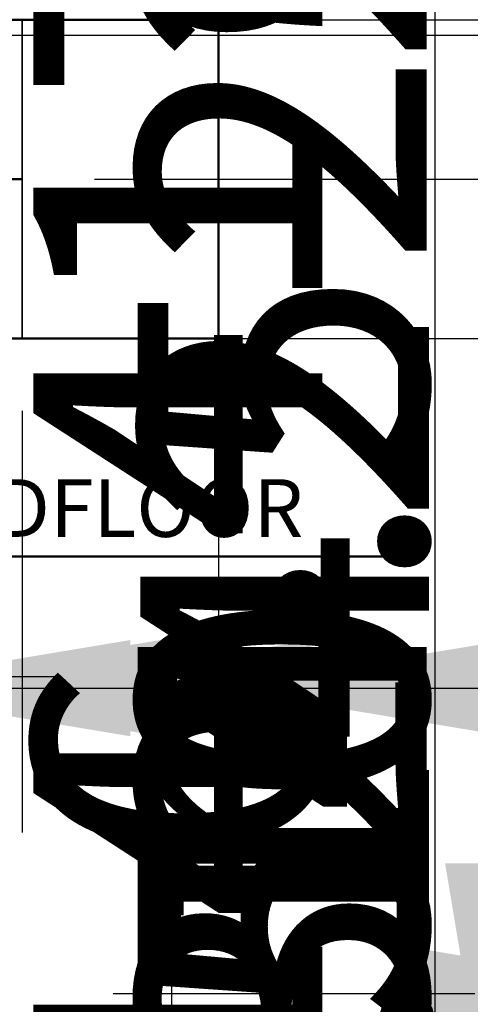
# Model space of a CAD drawing. Units: metres. Extents: x 782 to 1487, y 1262 to 7446.
# Tile 10 of 25: x 830.694 to 834.592, y 1284.539 to 1293.067. Entities that reach past the tile are written whole.
import ezdxf

# ---------------------------------------------------------------- set-up
doc = ezdxf.new("R2010")
doc.units = ezdxf.units.M
for name, color, linetype, lineweight in [('A-ANNO-DIMS', 2, 'Continuous', 18), ('A-ANNO-TEXT', 3, 'Continuous', 18), ('A-FLOR-STRS', 3, 'Continuous', 25), ('A-WALL', 7, 'Continuous', 50)]:
    doc.layers.add(name, color=color, linetype=linetype, lineweight=lineweight)
doc.styles.get("Standard").update_dxf_attribs({"font": 'arial.ttf'})
doc.dimstyles.new('ISO-25', dxfattribs={"dimtxt": 2.5, "dimasz": 2.5, "dimexe": 1.25, "dimexo": 0.625, "dimtad": 1, "dimtxsty": 'Standard', "dimcen": 2.5, "dimadec": 0, "dimazin": 0, "dimtfac": 1, "dimtmove": 0, "dimatfit": 3, "dimfxl": 1, "dimarcsym": 0})

# ---------------------------------------------------------------- blocks, each defined once
blk = doc.blocks.new('*D6')
at = {"layer": 'A-ANNO-DIMS', "color": 0, "lineweight": -2, "transparency": 16777216}
for p, q in [((833.0375, 1307.3274), (836.7683, 1307.3274)), ((835.5183, 1304.8274), (835.5183, 1295.5674)), ((833.0375, 1293.0674), (836.7683, 1293.0674))]:
    blk.add_line(p, q, dxfattribs=at)
at = {"layer": 'A-ANNO-DIMS', "color": 0, "transparency": 16777216}
for points in [[(835.1017, 1304.8274), (835.935, 1304.8274), (835.5183, 1307.3274)], [(835.1017, 1295.5674), (835.935, 1295.5674), (835.5183, 1293.0674)]]:
    blk.add_solid(points, dxfattribs=at)
at = {"layer": 'Defpoints', "color": 0, "transparency": 16777216}
for p in [(832.4125, 1307.3274), (832.4125, 1293.0674), (835.5183, 1293.0674)]:
    blk.add_point(p, dxfattribs=at)
at = {"layer": 'A-ANNO-DIMS', "color": 0, "transparency": 16777216, "insert": (833.3909, 1300.1974), "char_height": 2.5, "attachment_point": 5, "rotation": 90}
blk.add_mtext('14,26', dxfattribs=at)
blk = doc.blocks.new('*D22')
at = {"layer": 'A-ANNO-DIMS', "color": 0, "lineweight": -2, "transparency": 16777216}
for p, q in [((812.7897, 1292.934), (810.2897, 1292.934)), ((815.2897, 1292.934), (816.1792, 1292.934)), ((818.6792, 1292.934), (848.8344, 1292.934)), ((815.2897, 1292.4424), (815.2897, 1291.684)), ((816.1792, 1292.4424), (816.1792, 1291.684))]:
    blk.add_line(p, q, dxfattribs=at)
at = {"layer": 'A-ANNO-DIMS', "color": 0, "transparency": 16777216}
for points in [[(812.7897, 1293.3507), (812.7897, 1292.5173), (815.2897, 1292.934)], [(818.6792, 1293.3507), (818.6792, 1292.5173), (816.1792, 1292.934)]]:
    blk.add_solid(points, dxfattribs=at)
at = {"layer": 'Defpoints', "color": 0, "transparency": 16777216}
for p in [(815.2897, 1293.0674), (816.1792, 1293.0674), (816.1792, 1292.934)]:
    blk.add_point(p, dxfattribs=at)
at = {"layer": 'A-ANNO-DIMS', "color": 0, "transparency": 16777216, "insert": (835.0068, 1294.8525), "char_height": 2.5, "attachment_point": 5}
blk.add_mtext('DOOR 0.89 TYP.', dxfattribs=at)
blk = doc.blocks.new('*D24')
at = {"layer": 'A-ANNO-DIMS', "color": 0, "lineweight": -2, "transparency": 16777216}
for p, q in [((811.2086, 1294.4231), (808.7086, 1294.4231)), ((813.7086, 1294.4231), (814.5592, 1294.4231)), ((817.0592, 1294.4231), (852.6493, 1294.4231)), ((813.7086, 1293.9257), (813.7086, 1293.1731)), ((814.5592, 1293.9257), (814.5592, 1293.1731))]:
    blk.add_line(p, q, dxfattribs=at)
at = {"layer": 'A-ANNO-DIMS', "color": 0, "transparency": 16777216}
for points in [[(811.2086, 1294.8398), (811.2086, 1294.0065), (813.7086, 1294.4231)], [(817.0592, 1294.8398), (817.0592, 1294.0065), (814.5592, 1294.4231)]]:
    blk.add_solid(points, dxfattribs=at)
at = {"layer": 'Defpoints', "color": 0, "transparency": 16777216}
for p in [(813.7086, 1294.5507), (814.5592, 1294.5507), (814.5592, 1294.4231)]:
    blk.add_point(p, dxfattribs=at)
at = {"layer": 'A-ANNO-DIMS', "color": 0, "transparency": 16777216, "insert": (836.1042, 1296.3416), "char_height": 2.5, "attachment_point": 5}
blk.add_mtext('DOOR D2 0.85 TYP.', dxfattribs=at)
blk = doc.blocks.new('*D76')
at = {"layer": 'A-ANNO-DIMS', "color": 0, "lineweight": -2, "transparency": 16777216}
for p, q in [((814.8832, 1289.6803), (814.8832, 1286.127)), ((816.58, 1289.6803), (816.58, 1286.127)), ((812.3832, 1287.377), (809.8832, 1287.377)), ((814.8832, 1287.377), (816.58, 1287.377)), ((819.08, 1287.377), (831.0309, 1287.377))]:
    blk.add_line(p, q, dxfattribs=at)
at = {"layer": 'A-ANNO-DIMS', "color": 0, "transparency": 16777216}
for points in [[(812.3832, 1287.7936), (812.3832, 1286.9603), (814.8832, 1287.377)], [(819.08, 1287.7936), (819.08, 1286.9603), (816.58, 1287.377)]]:
    blk.add_solid(points, dxfattribs=at)
at = {"layer": 'Defpoints', "color": 0, "transparency": 16777216}
for p in [(814.8832, 1290.3053), (816.58, 1290.3053), (816.58, 1287.377)]:
    blk.add_point(p, dxfattribs=at)
at = {"layer": 'A-ANNO-DIMS', "color": 0, "transparency": 16777216, "insert": (826.3055, 1289.2784), "char_height": 2.5, "attachment_point": 5}
blk.add_mtext('1.697', dxfattribs=at)
blk = doc.blocks.new('*D87')
at = {"layer": 'A-ANNO-DIMS', "color": 0, "lineweight": -2, "transparency": 16777216}
for p, q in [((835.1905, 1309.8274), (835.1905, 1312.3274)), ((833.0375, 1307.3274), (836.4405, 1307.3274)), ((835.1905, 1307.3274), (835.1905, 1304.8669)), ((833.0382, 1304.8669), (836.4405, 1304.8669)), ((835.1905, 1302.3669), (835.1905, 1292.0821))]:
    blk.add_line(p, q, dxfattribs=at)
at = {"layer": 'A-ANNO-DIMS', "color": 0, "transparency": 16777216}
for points in [[(834.7738, 1309.8274), (835.6071, 1309.8274), (835.1905, 1307.3274)], [(834.7738, 1302.3669), (835.6071, 1302.3669), (835.1905, 1304.8669)]]:
    blk.add_solid(points, dxfattribs=at)
at = {"layer": 'Defpoints', "color": 0, "transparency": 16777216}
for p in [(832.4125, 1307.3274), (832.4132, 1304.8669), (835.1905, 1304.8669)]:
    blk.add_point(p, dxfattribs=at)
at = {"layer": 'A-ANNO-DIMS', "color": 0, "transparency": 16777216, "insert": (833.289, 1295.9745), "char_height": 2.5, "attachment_point": 5, "rotation": 90}
blk.add_mtext('2.46', dxfattribs=at)
blk = doc.blocks.new('*D88')
at = {"layer": 'A-ANNO-DIMS', "color": 0, "lineweight": -2, "transparency": 16777216}
for p, q in [((835.1905, 1307.3669), (835.1905, 1309.8669)), ((833.0382, 1304.8669), (836.4405, 1304.8669)), ((835.1905, 1304.8669), (835.1905, 1300.3378)), ((833.0381, 1300.3378), (836.4405, 1300.3378)), ((835.1905, 1297.8378), (835.1905, 1285.5459))]:
    blk.add_line(p, q, dxfattribs=at)
at = {"layer": 'A-ANNO-DIMS', "color": 0, "transparency": 16777216}
for points in [[(834.7738, 1307.3669), (835.6071, 1307.3669), (835.1905, 1304.8669)], [(834.7738, 1297.8378), (835.6071, 1297.8378), (835.1905, 1300.3378)]]:
    blk.add_solid(points, dxfattribs=at)
at = {"layer": 'Defpoints', "color": 0, "transparency": 16777216}
for p in [(832.4132, 1304.8669), (832.4131, 1300.3378), (835.1905, 1300.3378)]:
    blk.add_point(p, dxfattribs=at)
at = {"layer": 'A-ANNO-DIMS', "color": 0, "transparency": 16777216, "insert": (833.289, 1290.4419), "char_height": 2.5, "attachment_point": 5, "rotation": 90}
blk.add_mtext('4.529', dxfattribs=at)
blk = doc.blocks.new('*D89')
at = {"layer": 'A-ANNO-DIMS', "color": 0, "lineweight": -2, "transparency": 16777216}
for p, q in [((835.1905, 1302.8378), (835.1905, 1305.3378)), ((833.0381, 1300.3378), (836.4405, 1300.3378)), ((835.1905, 1300.3378), (835.1905, 1296.196)), ((833.0375, 1296.196), (836.4405, 1296.196)), ((835.1905, 1293.696), (835.1905, 1281.4347))]:
    blk.add_line(p, q, dxfattribs=at)
at = {"layer": 'A-ANNO-DIMS', "color": 0, "transparency": 16777216}
for points in [[(834.7738, 1302.8378), (835.6071, 1302.8378), (835.1905, 1300.3378)], [(834.7738, 1293.696), (835.6071, 1293.696), (835.1905, 1296.196)]]:
    blk.add_solid(points, dxfattribs=at)
at = {"layer": 'Defpoints', "color": 0, "transparency": 16777216}
for p in [(832.4131, 1300.3378), (832.4125, 1296.196), (835.1905, 1296.196)]:
    blk.add_point(p, dxfattribs=at)
at = {"layer": 'A-ANNO-DIMS', "color": 0, "transparency": 16777216, "insert": (833.3103, 1286.3153), "char_height": 2.5, "attachment_point": 5, "rotation": 90}
blk.add_mtext('4.142', dxfattribs=at)
blk = doc.blocks.new('*D90')
at = {"layer": 'A-ANNO-DIMS', "color": 0, "lineweight": -2, "transparency": 16777216}
for p, q in [((835.1905, 1298.696), (835.1905, 1301.196)), ((833.0375, 1296.196), (836.4405, 1296.196)), ((835.1905, 1296.196), (835.1905, 1293.6994)), ((833.0375, 1293.6994), (836.4405, 1293.6994)), ((835.1905, 1291.1994), (835.1905, 1280.9214))]:
    blk.add_line(p, q, dxfattribs=at)
at = {"layer": 'A-ANNO-DIMS', "color": 0, "transparency": 16777216}
for points in [[(834.7738, 1298.696), (835.6071, 1298.696), (835.1905, 1296.196)], [(834.7738, 1291.1994), (835.6071, 1291.1994), (835.1905, 1293.6994)]]:
    blk.add_solid(points, dxfattribs=at)
at = {"layer": 'Defpoints', "color": 0, "transparency": 16777216}
for p in [(832.4125, 1296.196), (832.4125, 1293.6994), (835.1905, 1293.6994)]:
    blk.add_point(p, dxfattribs=at)
at = {"layer": 'A-ANNO-DIMS', "color": 0, "transparency": 16777216, "insert": (833.289, 1284.8104), "char_height": 2.5, "attachment_point": 5, "rotation": 90}
blk.add_mtext('2.50', dxfattribs=at)
blk = doc.blocks.new('*D91')
at = {"layer": 'A-ANNO-DIMS', "color": 0, "lineweight": -2, "transparency": 16777216}
for p, q in [((835.1905, 1296.1994), (835.1905, 1298.6994)), ((833.0375, 1293.6994), (836.4405, 1293.6994)), ((835.1905, 1293.6994), (835.1905, 1293.0674)), ((833.0375, 1293.0674), (836.4405, 1293.0674)), ((835.1905, 1290.5674), (835.1905, 1278.4068))]:
    blk.add_line(p, q, dxfattribs=at)
at = {"layer": 'A-ANNO-DIMS', "color": 0, "transparency": 16777216}
for points in [[(834.7738, 1296.1994), (835.6071, 1296.1994), (835.1905, 1293.6994)], [(834.7738, 1290.5674), (835.6071, 1290.5674), (835.1905, 1293.0674)]]:
    blk.add_solid(points, dxfattribs=at)
at = {"layer": 'Defpoints', "color": 0, "transparency": 16777216}
for p in [(832.4125, 1293.6994), (832.4125, 1293.0674), (835.1905, 1293.0674)]:
    blk.add_point(p, dxfattribs=at)
at = {"layer": 'A-ANNO-DIMS', "color": 0, "transparency": 16777216, "insert": (833.2882, 1283.2371), "char_height": 2.5, "attachment_point": 5, "rotation": 90}
blk.add_mtext('0.632', dxfattribs=at)
blk = doc.blocks.new('*D92')
at = {"layer": 'A-ANNO-DIMS', "color": 0, "lineweight": -2, "transparency": 16777216}
for p, q in [((835.1905, 1295.5674), (835.1905, 1298.0674)), ((831.3406, 1293.0674), (836.4405, 1293.0674)), ((835.1905, 1293.0674), (835.1905, 1291.6863)), ((831.3406, 1291.6863), (836.4405, 1291.6863)), ((835.1905, 1289.1863), (835.1905, 1277.7181))]:
    blk.add_line(p, q, dxfattribs=at)
at = {"layer": 'A-ANNO-DIMS', "color": 0, "transparency": 16777216}
for points in [[(834.7738, 1295.5674), (835.6071, 1295.5674), (835.1905, 1293.0674)], [(834.7738, 1289.1863), (835.6071, 1289.1863), (835.1905, 1291.6863)]]:
    blk.add_solid(points, dxfattribs=at)
at = {"layer": 'Defpoints', "color": 0, "transparency": 16777216}
for p in [(830.7156, 1293.0674), (830.7156, 1291.6863), (835.1905, 1291.6863)]:
    blk.add_point(p, dxfattribs=at)
at = {"layer": 'A-ANNO-DIMS', "color": 0, "transparency": 16777216, "insert": (833.2882, 1282.2022), "char_height": 2.5, "attachment_point": 5, "rotation": 90}
blk.add_mtext('1.381', dxfattribs=at)
blk = doc.blocks.new('*D93')
at = {"layer": 'A-ANNO-DIMS', "color": 0, "lineweight": -2, "transparency": 16777216}
for p, q in [((835.1905, 1294.1863), (835.1905, 1296.6863)), ((831.3406, 1291.6863), (836.4405, 1291.6863)), ((835.1905, 1291.6863), (835.1905, 1290.3053)), ((831.3406, 1290.3053), (836.4405, 1290.3053)), ((835.1905, 1287.8053), (835.1905, 1276.337))]:
    blk.add_line(p, q, dxfattribs=at)
at = {"layer": 'A-ANNO-DIMS', "color": 0, "transparency": 16777216}
for points in [[(834.7738, 1294.1863), (835.6071, 1294.1863), (835.1905, 1291.6863)], [(834.7738, 1287.8053), (835.6071, 1287.8053), (835.1905, 1290.3053)]]:
    blk.add_solid(points, dxfattribs=at)
at = {"layer": 'Defpoints', "color": 0, "transparency": 16777216}
for p in [(830.7156, 1291.6863), (830.7156, 1290.3053), (835.1905, 1290.3053)]:
    blk.add_point(p, dxfattribs=at)
at = {"layer": 'A-ANNO-DIMS', "color": 0, "transparency": 16777216, "insert": (833.2882, 1280.8211), "char_height": 2.5, "attachment_point": 5, "rotation": 90}
blk.add_mtext('1.381', dxfattribs=at)
blk = doc.blocks.new('*D97')
at = {"layer": 'A-ANNO-DIMS', "color": 0, "lineweight": -2, "transparency": 16777216}
for p, q in [((827.9625, 1289.6803), (827.9625, 1286.0275)), ((829.1513, 1289.6803), (829.1513, 1286.0275)), ((825.4625, 1287.2775), (822.9625, 1287.2775)), ((827.9625, 1287.2775), (829.1513, 1287.2775)), ((831.6513, 1287.2775), (841.6649, 1287.2775))]:
    blk.add_line(p, q, dxfattribs=at)
at = {"layer": 'A-ANNO-DIMS', "color": 0, "transparency": 16777216}
for points in [[(825.4625, 1287.6941), (825.4625, 1286.8608), (827.9625, 1287.2775)], [(831.6513, 1287.6941), (831.6513, 1286.8608), (829.1513, 1287.2775)]]:
    blk.add_solid(points, dxfattribs=at)
at = {"layer": 'Defpoints', "color": 0, "transparency": 16777216}
for p in [(827.9625, 1290.3053), (829.1513, 1290.3053), (829.1513, 1287.2775)]:
    blk.add_point(p, dxfattribs=at)
at = {"layer": 'A-ANNO-DIMS', "color": 0, "transparency": 16777216, "insert": (837.9081, 1289.1789), "char_height": 2.5, "attachment_point": 5}
blk.add_mtext('1.19', dxfattribs=at)
blk = doc.blocks.new('*D98')
at = {"layer": 'A-ANNO-DIMS', "color": 0, "lineweight": -2, "transparency": 16777216}
for p, q in [((829.1513, 1289.6803), (829.1513, 1286.0275)), ((829.412, 1289.6803), (829.412, 1286.0275)), ((826.6513, 1287.2775), (824.1513, 1287.2775)), ((829.1513, 1287.2775), (829.412, 1287.2775)), ((831.912, 1287.2775), (842.1542, 1287.2775))]:
    blk.add_line(p, q, dxfattribs=at)
at = {"layer": 'A-ANNO-DIMS', "color": 0, "transparency": 16777216}
for points in [[(826.6513, 1287.6941), (826.6513, 1286.8608), (829.1513, 1287.2775)], [(831.912, 1287.6941), (831.912, 1286.8608), (829.412, 1287.2775)]]:
    blk.add_solid(points, dxfattribs=at)
at = {"layer": 'Defpoints', "color": 0, "transparency": 16777216}
for p in [(829.1513, 1290.3053), (829.412, 1290.3053), (829.412, 1287.2775)]:
    blk.add_point(p, dxfattribs=at)
at = {"layer": 'A-ANNO-DIMS', "color": 0, "transparency": 16777216, "insert": (838.2831, 1289.1789), "char_height": 2.5, "attachment_point": 5}
blk.add_mtext('0.26', dxfattribs=at)
blk = doc.blocks.new('*D99')
at = {"layer": 'A-ANNO-DIMS', "color": 0, "lineweight": -2, "transparency": 16777216}
for p, q in [((829.412, 1289.6803), (829.412, 1286.0275)), ((830.7156, 1289.6803), (830.7156, 1286.0275)), ((826.912, 1287.2775), (824.412, 1287.2775)), ((829.412, 1287.2775), (830.7156, 1287.2775)), ((833.2156, 1287.2775), (843.2156, 1287.2775))]:
    blk.add_line(p, q, dxfattribs=at)
at = {"layer": 'A-ANNO-DIMS', "color": 0, "transparency": 16777216}
for points in [[(826.912, 1287.6941), (826.912, 1286.8608), (829.412, 1287.2775)], [(833.2156, 1287.6941), (833.2156, 1286.8608), (830.7156, 1287.2775)]]:
    blk.add_solid(points, dxfattribs=at)
at = {"layer": 'Defpoints', "color": 0, "transparency": 16777216}
for p in [(829.412, 1290.3053), (830.7156, 1290.3053), (830.7156, 1287.2775)]:
    blk.add_point(p, dxfattribs=at)
at = {"layer": 'A-ANNO-DIMS', "color": 0, "transparency": 16777216, "insert": (839.4656, 1289.1798), "char_height": 2.5, "attachment_point": 5}
blk.add_mtext('1.30', dxfattribs=at)
blk = doc.blocks.new('*D100')
at = {"layer": 'A-ANNO-DIMS', "color": 0, "lineweight": -2, "transparency": 16777216}
for p, q in [((830.7156, 1289.6803), (830.7156, 1286.0275)), ((832.4125, 1289.6803), (832.4125, 1286.0275)), ((828.2156, 1287.2775), (825.7156, 1287.2775)), ((830.7156, 1287.2775), (832.4125, 1287.2775)), ((834.9125, 1287.2775), (846.8634, 1287.2775))]:
    blk.add_line(p, q, dxfattribs=at)
at = {"layer": 'A-ANNO-DIMS', "color": 0, "transparency": 16777216}
for points in [[(828.2156, 1287.6941), (828.2156, 1286.8608), (830.7156, 1287.2775)], [(834.9125, 1287.6941), (834.9125, 1286.8608), (832.4125, 1287.2775)]]:
    blk.add_solid(points, dxfattribs=at)
at = {"layer": 'Defpoints', "color": 0, "transparency": 16777216}
for p in [(830.7156, 1290.3053), (832.4125, 1290.3053), (832.4125, 1287.2775)]:
    blk.add_point(p, dxfattribs=at)
at = {"layer": 'A-ANNO-DIMS', "color": 0, "transparency": 16777216, "insert": (842.1379, 1289.1789), "char_height": 2.5, "attachment_point": 5}
blk.add_mtext('1.697', dxfattribs=at)
blk = doc.blocks.new('*D154')
at = {"layer": 'A-ANNO-DIMS', "color": 0, "lineweight": -2, "transparency": 16777216}
for p, q in [((834.2886, 1275.5562), (834.2886, 1287.7305)), ((836.1342, 1273.0562), (833.0386, 1273.0562)), ((834.2886, 1269.1422), (834.2886, 1273.0562)), ((836.1187, 1269.1422), (833.0386, 1269.1422)), ((834.2886, 1266.6422), (834.2886, 1264.1422))]:
    blk.add_line(p, q, dxfattribs=at)
at = {"layer": 'A-ANNO-DIMS', "color": 0, "transparency": 16777216}
for points in [[(833.8719, 1275.5562), (834.7052, 1275.5562), (834.2886, 1273.0562)], [(833.8719, 1266.6422), (834.7052, 1266.6422), (834.2886, 1269.1422)]]:
    blk.add_solid(points, dxfattribs=at)
at = {"layer": 'Defpoints', "color": 0, "transparency": 16777216}
for p in [(834.2886, 1273.0562), (836.7592, 1273.0562), (836.7437, 1269.1422)]:
    blk.add_point(p, dxfattribs=at)
at = {"layer": 'A-ANNO-DIMS', "color": 0, "transparency": 16777216, "insert": (832.3863, 1282.8934), "char_height": 2.5, "attachment_point": 5, "rotation": 90}
blk.add_mtext('3.914', dxfattribs=at)
blk = doc.blocks.new('*D157')
at = {"layer": 'A-ANNO-DIMS', "color": 0, "lineweight": -2, "transparency": 16777216}
for p, q in [((834.2886, 1282.619), (834.2886, 1294.8189)), ((835.8783, 1282.619), (833.0386, 1282.619)), ((834.2886, 1278.7022), (834.2886, 1280.119)), ((835.8783, 1276.2022), (833.0386, 1276.2022))]:
    blk.add_line(p, q, dxfattribs=at)
at = {"layer": 'A-ANNO-DIMS', "color": 0, "transparency": 16777216}
for points in [[(833.8719, 1280.119), (834.7052, 1280.119), (834.2886, 1282.619)], [(833.8719, 1278.7022), (834.7052, 1278.7022), (834.2886, 1276.2022)]]:
    blk.add_solid(points, dxfattribs=at)
at = {"layer": 'Defpoints', "color": 0, "transparency": 16777216}
for p in [(834.2886, 1282.619), (836.5033, 1282.619), (836.5033, 1276.2022)]:
    blk.add_point(p, dxfattribs=at)
at = {"layer": 'A-ANNO-DIMS', "color": 0, "transparency": 16777216, "insert": (832.3871, 1289.9689), "char_height": 2.5, "attachment_point": 5, "rotation": 90}
blk.add_mtext('6.417', dxfattribs=at)
blk = doc.blocks.new('*D158')
at = {"layer": 'A-ANNO-DIMS', "color": 0, "lineweight": -2, "transparency": 16777216}
for p, q in [((836.5033, 1283.244), (836.5033, 1285.8791)), ((837.1321, 1282.6436), (837.1321, 1285.8791)), ((834.0033, 1284.6291), (831.5033, 1284.6291)), ((836.5033, 1284.6291), (837.1321, 1284.6291)), ((839.6321, 1284.6291), (849.876, 1284.6291))]:
    blk.add_line(p, q, dxfattribs=at)
at = {"layer": 'A-ANNO-DIMS', "color": 0, "transparency": 16777216}
for points in [[(834.0033, 1285.0458), (834.0033, 1284.2125), (836.5033, 1284.6291)], [(839.6321, 1285.0458), (839.6321, 1284.2125), (837.1321, 1284.6291)]]:
    blk.add_solid(points, dxfattribs=at)
at = {"layer": 'Defpoints', "color": 0, "transparency": 16777216}
for p in [(837.1321, 1284.6291), (836.5033, 1282.619), (837.1321, 1282.0186)]:
    blk.add_point(p, dxfattribs=at)
at = {"layer": 'A-ANNO-DIMS', "color": 0, "transparency": 16777216, "insert": (846.004, 1286.5314), "char_height": 2.5, "attachment_point": 5}
blk.add_mtext('0.63', dxfattribs=at)
blk = doc.blocks.new('*D159')
at = {"layer": 'A-ANNO-DIMS', "color": 0, "lineweight": -2, "transparency": 16777216}
for p, q in [((837.1321, 1282.6436), (837.1321, 1285.8791)), ((839.8262, 1282.6436), (839.8262, 1285.8791)), ((834.6321, 1284.6291), (832.1321, 1284.6291)), ((837.1321, 1284.6291), (839.8262, 1284.6291)), ((842.3262, 1284.6291), (854.5449, 1284.6291))]:
    blk.add_line(p, q, dxfattribs=at)
at = {"layer": 'A-ANNO-DIMS', "color": 0, "transparency": 16777216}
for points in [[(834.6321, 1285.0458), (834.6321, 1284.2125), (837.1321, 1284.6291)], [(842.3262, 1285.0458), (842.3262, 1284.2125), (839.8262, 1284.6291)]]:
    blk.add_solid(points, dxfattribs=at)
at = {"layer": 'Defpoints', "color": 0, "transparency": 16777216}
for p in [(839.8262, 1284.6291), (837.1321, 1282.0186), (839.8262, 1282.0186)]:
    blk.add_point(p, dxfattribs=at)
at = {"layer": 'A-ANNO-DIMS', "color": 0, "transparency": 16777216, "insert": (849.6855, 1286.5306), "char_height": 2.5, "attachment_point": 5}
blk.add_mtext('2.694', dxfattribs=at)
blk = doc.blocks.new('*D165')
at = {"layer": 'A-ANNO-DIMS', "color": 0, "lineweight": -2, "transparency": 16777216}
for p, q in [((826.3877, 1283.8847), (826.3877, 1285.3747)), ((832.0105, 1283.8847), (832.0105, 1285.3747)), ((823.8877, 1284.1247), (821.3877, 1284.1247)), ((826.3877, 1284.1247), (832.0105, 1284.1247)), ((834.5105, 1284.1247), (846.6967, 1284.1247))]:
    blk.add_line(p, q, dxfattribs=at)
at = {"layer": 'A-ANNO-DIMS', "color": 0, "transparency": 16777216}
for points in [[(823.8877, 1284.5413), (823.8877, 1283.708), (826.3877, 1284.1247)], [(834.5105, 1284.5413), (834.5105, 1283.708), (832.0105, 1284.1247)]]:
    blk.add_solid(points, dxfattribs=at)
at = {"layer": 'Defpoints', "color": 0, "transparency": 16777216}
for p in [(832.0105, 1284.1247), (826.3877, 1283.2597), (832.0105, 1283.2597)]:
    blk.add_point(p, dxfattribs=at)
at = {"layer": 'A-ANNO-DIMS', "color": 0, "transparency": 16777216, "insert": (841.8536, 1286.027), "char_height": 2.5, "attachment_point": 5}
blk.add_mtext('5.623', dxfattribs=at)
blk = doc.blocks.new('*D167')
at = {"layer": 'A-ANNO-DIMS', "color": 0, "lineweight": -2, "transparency": 16777216}
for p, q in [((834.7907, 1285.7597), (834.7907, 1288.2597)), ((832.6355, 1283.2597), (836.0407, 1283.2597)), ((834.7907, 1283.2597), (834.7907, 1282.1784)), ((831.7457, 1282.1784), (836.0407, 1282.1784)), ((834.7907, 1279.6784), (834.7907, 1269.6648))]:
    blk.add_line(p, q, dxfattribs=at)
at = {"layer": 'A-ANNO-DIMS', "color": 0, "transparency": 16777216}
for points in [[(834.3741, 1285.7597), (835.2074, 1285.7597), (834.7907, 1283.2597)], [(834.3741, 1279.6784), (835.2074, 1279.6784), (834.7907, 1282.1784)]]:
    blk.add_solid(points, dxfattribs=at)
at = {"layer": 'Defpoints', "color": 0, "transparency": 16777216}
for p in [(832.0105, 1283.2597), (831.1207, 1282.1784), (834.7907, 1282.1784)]:
    blk.add_point(p, dxfattribs=at)
at = {"layer": 'A-ANNO-DIMS', "color": 0, "transparency": 16777216, "insert": (832.8893, 1273.4216), "char_height": 2.5, "attachment_point": 5, "rotation": 90}
blk.add_mtext('1.08', dxfattribs=at)
blk = doc.blocks.new('*D168')
at = {"layer": 'A-ANNO-DIMS', "color": 0, "lineweight": -2, "transparency": 16777216}
for p, q in [((834.7907, 1284.6784), (834.7907, 1287.1784)), ((831.7457, 1282.1784), (836.0407, 1282.1784)), ((834.7907, 1282.1784), (834.7907, 1279.1214)), ((831.7457, 1279.1214), (836.0407, 1279.1214)), ((834.7907, 1276.6214), (834.7907, 1264.4369))]:
    blk.add_line(p, q, dxfattribs=at)
at = {"layer": 'A-ANNO-DIMS', "color": 0, "transparency": 16777216}
for points in [[(834.3741, 1284.6784), (835.2074, 1284.6784), (834.7907, 1282.1784)], [(834.3741, 1276.6214), (835.2074, 1276.6214), (834.7907, 1279.1214)]]:
    blk.add_solid(points, dxfattribs=at)
at = {"layer": 'Defpoints', "color": 0, "transparency": 16777216}
for p in [(831.1207, 1282.1784), (831.1207, 1279.1214), (834.7907, 1279.1214)]:
    blk.add_point(p, dxfattribs=at)
at = {"layer": 'A-ANNO-DIMS', "color": 0, "transparency": 16777216, "insert": (832.8885, 1269.2791), "char_height": 2.5, "attachment_point": 5, "rotation": 90}
blk.add_mtext('3.057', dxfattribs=at)

msp = doc.modelspace()

# ---------------------------------------------------------------- linework, layer by layer
at = {"layer": 'A-FLOR-STRS'}
for p, q in [((830.7156, 1290.3053), (830.7156, 1293.0674)), ((830.7156, 1293.0674), (830.7156, 1290.3053)), ((830.7156, 1293.0674), (830.7156, 1291.6863)), ((830.7156, 1290.3053), (830.7156, 1291.6863))]:
    msp.add_line(p, q, dxfattribs=at)
at = {"layer": 'A-WALL'}
for p, q in [((832.4125, 1303.3374), (832.4125, 1293.0674)), ((832.4125, 1293.0674), (827.9625, 1293.0674)), ((830.6725, 1293.0674), (831.1618, 1293.0674)), ((831.9738, 1293.0674), (832.4125, 1293.0674)), ((832.0625, 1293.0674), (832.0117, 1293.0674)), ((832.4125, 1290.3053), (832.4125, 1293.0674)), ((830.7156, 1291.6863), (827.9625, 1291.6863)), ((830.7156, 1291.6863), (827.9625, 1291.6863)), ((827.9625, 1290.3053), (832.4125, 1290.3053)), ((828.0178, 1288.4175), (834.0505, 1288.4175))]:
    msp.add_line(p, q, dxfattribs=at)

# ---------------------------------------------------------------- texts
at = {"layer": 'A-ANNO-TEXT', "insert": (828.2435, 1289.921), "char_height": 0.5, "attachment_point": 1}
msp.add_mtext_dynamic_manual_height_columns('\\PSECONDFLOOR', width=4.240641, gutter_width=12.5, heights=[0], dxfattribs=at)

# ---------------------------------------------------------------- dimensions: what is measured, and where the dimension line sits
at = {"layer": 'A-ANNO-DIMS'}
for base, p1, p2, override, picture, middle in [((835.1905, 1304.8669), (832.4125, 1307.3274), (832.4132, 1304.8669), {"dimdec": 2, "dimlfac": 1, "dimrnd": 0, "dimzin": 0, "dimdsep": 46, "dimlunit": 2}, '*D87', (833.289, 1295.9745)), ((835.1905, 1300.3378), (832.4132, 1304.8669), (832.4131, 1300.3378), {"dimdec": 3, "dimlfac": 1, "dimrnd": 0, "dimzin": 0, "dimdsep": 46, "dimlunit": 2}, '*D88', (833.289, 1290.4419)), ((835.5183, 1293.0674), (832.4125, 1307.3274), (832.4125, 1293.0674), {"dimclrd": 0, "dimclre": 0, "dimclrt": 0}, '*D6', (833.3909, 1300.1974)), ((835.1905, 1296.196), (832.4131, 1300.3378), (832.4125, 1296.196), {"dimdec": 3, "dimlfac": 1, "dimrnd": 0, "dimzin": 0, "dimdsep": 46, "dimlunit": 2}, '*D89', (833.3103, 1286.3153)), ((835.1905, 1293.6994), (832.4125, 1296.196), (832.4125, 1293.6994), {"dimdec": 2, "dimlfac": 1, "dimrnd": 0, "dimzin": 0, "dimdsep": 46, "dimlunit": 2}, '*D90', (833.289, 1284.8104)), ((835.1905, 1293.0674), (832.4125, 1293.6994), (832.4125, 1293.0674), {"dimdec": 3, "dimlfac": 1, "dimrnd": 0, "dimzin": 0, "dimdsep": 46, "dimlunit": 2}, '*D91', (833.2882, 1283.2371)), ((835.1905, 1291.6863), (830.7156, 1293.0674), (830.7156, 1291.6863), {"dimdec": 3, "dimlfac": 1, "dimrnd": 0, "dimzin": 0, "dimdsep": 46, "dimlunit": 2}, '*D92', (833.2882, 1282.2022)), ((835.1905, 1290.3053), (830.7156, 1291.6863), (830.7156, 1290.3053), {"dimdec": 3, "dimlfac": 1, "dimrnd": 0, "dimzin": 0, "dimdsep": 46, "dimlunit": 2}, '*D93', (833.2882, 1280.8211)), ((834.2886, 1282.619), (836.5033, 1276.2022), (836.5033, 1282.619), {"dimdec": 3, "dimlfac": 1, "dimrnd": 0, "dimzin": 0, "dimdsep": 46, "dimlunit": 2}, '*D157', (832.3871, 1289.9689)), ((834.7907, 1282.1784), (832.0105, 1283.2597), (831.1207, 1282.1784), {"dimdec": 2, "dimlfac": 1, "dimrnd": 0, "dimzin": 0, "dimdsep": 46, "dimlunit": 2}, '*D167', (832.8893, 1273.4216)), ((834.2886, 1273.0562), (836.7437, 1269.1422), (836.7592, 1273.0562), {"dimdec": 3, "dimlfac": 1, "dimrnd": 0, "dimzin": 0, "dimdsep": 46, "dimlunit": 2}, '*D154', (832.3863, 1282.8934)), ((834.7907, 1279.1214), (831.1207, 1282.1784), (831.1207, 1279.1214), {"dimdec": 3, "dimlfac": 1, "dimrnd": 0, "dimzin": 0, "dimdsep": 46, "dimlunit": 2}, '*D168', (832.8885, 1269.2791))]:
    dim = msp.add_linear_dim(base=base, p1=p1, p2=p2, angle=90, dimstyle='ISO-25', override=override, dxfattribs=at)
    dim.commit()
    dim.dimension.update_dxf_attribs({"geometry": picture, "text_midpoint": middle})
for base, p1, p2, text, picture, middle in [((814.5592, 1294.4231), (813.7086, 1294.5507), (814.5592, 1294.5507), 'DOOR D2 <> TYP.', '*D24', (836.1042, 1296.3416)), ((816.1792, 1292.934), (815.2897, 1293.0674), (816.1792, 1293.0674), 'DOOR <> TYP.', '*D22', (835.0068, 1294.8525))]:
    dim = msp.add_linear_dim(base=base, p1=p1, p2=p2, text=text, dimstyle='ISO-25', override={"dimdec": 2, "dimlfac": 1, "dimrnd": 0, "dimzin": 0, "dimdsep": 46, "dimlunit": 2}, dxfattribs=at)
    dim.commit()
    dim.dimension.update_dxf_attribs({"geometry": picture, "text_midpoint": middle})
for base, p1, p2, override, picture, middle in [((816.58, 1287.377), (814.8832, 1290.3053), (816.58, 1290.3053), {"dimdec": 3, "dimlfac": 1, "dimrnd": 0, "dimzin": 0, "dimdsep": 46, "dimlunit": 2}, '*D76', (826.3055, 1289.2784)), ((829.1513, 1287.2775), (827.9625, 1290.3053), (829.1513, 1290.3053), {"dimdec": 2, "dimlfac": 1, "dimrnd": 0, "dimzin": 0, "dimdsep": 46, "dimlunit": 2}, '*D97', (837.9081, 1289.1789)), ((829.412, 1287.2775), (829.1513, 1290.3053), (829.412, 1290.3053), {"dimdec": 2, "dimlfac": 1, "dimrnd": 0, "dimzin": 0, "dimdsep": 46, "dimlunit": 2}, '*D98', (838.2831, 1289.1789)), ((830.7156, 1287.2775), (829.412, 1290.3053), (830.7156, 1290.3053), {"dimdec": 2, "dimlfac": 1, "dimrnd": 0, "dimzin": 0, "dimdsep": 46, "dimlunit": 2}, '*D99', (839.4656, 1289.1798)), ((832.4125, 1287.2775), (830.7156, 1290.3053), (832.4125, 1290.3053), {"dimdec": 3, "dimlfac": 1, "dimrnd": 0, "dimzin": 0, "dimdsep": 46, "dimlunit": 2}, '*D100', (842.1379, 1289.1789)), ((837.1321, 1284.6291), (836.5033, 1282.619), (837.1321, 1282.0186), {"dimdec": 2, "dimlfac": 1, "dimrnd": 0, "dimzin": 0, "dimdsep": 46, "dimlunit": 2}, '*D158', (846.004, 1286.5314)), ((839.8262, 1284.6291), (837.1321, 1282.0186), (839.8262, 1282.0186), {"dimdec": 3, "dimlfac": 1, "dimrnd": 0, "dimzin": 0, "dimdsep": 46, "dimlunit": 2}, '*D159', (849.6855, 1286.5306)), ((832.0105, 1284.1247), (826.3877, 1283.2597), (832.0105, 1283.2597), {"dimdec": 3, "dimlfac": 1, "dimrnd": 0, "dimzin": 0, "dimdsep": 46, "dimlunit": 2}, '*D165', (841.8536, 1286.027))]:
    dim = msp.add_linear_dim(base=base, p1=p1, p2=p2, dimstyle='ISO-25', override=override, dxfattribs=at)
    dim.commit()
    dim.dimension.update_dxf_attribs({"geometry": picture, "text_midpoint": middle})

doc.saveas('drawing.dxf')
